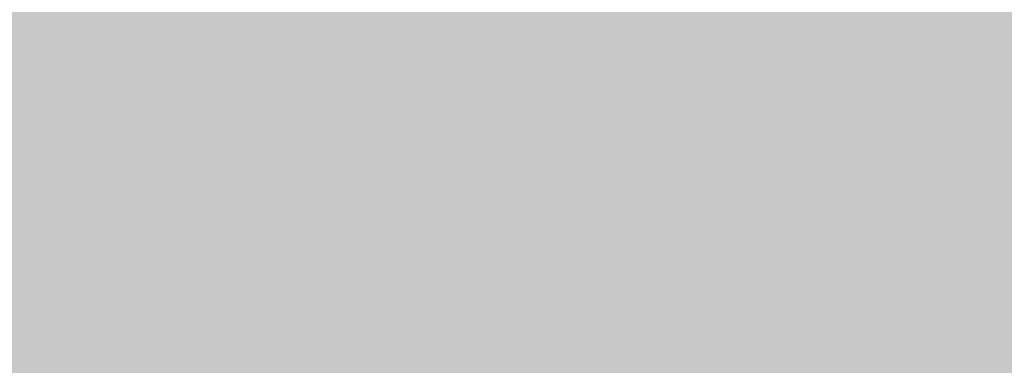
# Model space of a CAD drawing. Units: inches. Extents: x 2091 to 2899, y 967 to 2217.
# Tile 232 of 256: x 2203.4104 to 2203.7172, y 1152.3547 to 1152.4622. Entities that reach past the tile are written whole.
import ezdxf

# ---------------------------------------------------------------- set-up
doc = ezdxf.new("R2010")
doc.units = ezdxf.units.IN
doc.layers.add('A-WALL-PATT', color=141, linetype='Continuous', lineweight=13, true_color=0xadddf7)

msp = doc.modelspace()

# ---------------------------------------------------------------- hatches: boundary and pattern name
at = {"layer": 'A-WALL-PATT'}
h = msp.add_hatch(color=256, dxfattribs=at)
h.dxf.hatch_style = 1
h.paths.add_polyline_path([(2803.1436, 2050.91906), (2203.1436, 2050.91906), (2203.1436, 1090.91906), (2803.1436, 1090.91906)])
h.paths.add_polyline_path([(2635.79885, 1147.54046), (2674.52405, 1147.54046, 0.376086), (2678.52967, 1152.8802), (2678.52967, 1159.55647, 0.333335), (2674.52432, 1163.56185), (2674.52432, 1163.56185), (2674.52432, 1192.93439), (2635.80597, 1192.93439), (2597.08762, 1192.93439), (2597.08762, 1163.56185, 0.333335), (2593.08228, 1159.55647), (2593.08228, 1152.8802, 0.376086), (2597.08789, 1147.54046)], flags=0)
h.paths.add_polyline_path([(2436.01043, 1278.24078, 0.000483), (2435.95264, 1278.21503, -0.001328), (2435.93563, 1278.11169, -0.001711), (2436.11644, 1278.04076, 0.002185)], flags=0)
h.paths.add_polyline_path([(2794.1436, 1143.41906), (2794.1436, 1347.41906), (2543.37017, 1347.41906), (2543.37017, 1351.91906), (2794.1436, 1351.91906), (2794.1436, 1392.71355), (2793.9474, 1392.71355), (2793.9474, 1473.5369), (2794.1436, 1473.5369), (2794.1436, 1531.91906), (2650.1436, 1531.91906), (2650.1436, 1536.41906), (2794.1436, 1536.41906), (2794.1436, 1692.41906), (2609.37561, 1692.41906), (2609.37561, 1644.41906), (2604.87561, 1644.41906), (2604.87561, 1744.91906), (2609.37561, 1744.91906), (2609.37561, 1696.91906), (2794.1436, 1696.91906), (2794.1436, 1780.91906), (2609.6436, 1780.91906), (2493.87561, 1780.91906), (2493.87561, 1785.41906), (2609.6436, 1785.41906), (2794.1436, 1785.41906), (2794.1436, 1847.93882), (2793.95122, 1847.93882), (2793.95122, 1928.76217), (2794.1436, 1928.76217), (2794.1436, 1941.41906), (2614.1436, 1941.41906), (2614.1436, 1821.41906), (2609.6436, 1821.41906), (2609.6436, 1941.41906), (2392.1436, 1941.41906), (2392.1436, 1819.91906), (2387.6436, 1819.91906), (2387.6436, 1941.41906), (2212.1436, 1941.41906), (2212.1436, 1783.91906), (2392.1436, 1783.91906), (2392.1436, 1780.91906), (2212.1436, 1780.91906), (2212.1436, 1629.41906), (2387.6436, 1629.41906), (2387.6436, 1744.91906), (2392.1436, 1744.91906), (2392.1436, 1627.91906), (2317.1436, 1627.91906), (2317.1436, 1551.41906), (2317.1436, 1536.41906), (2459.38359, 1536.41906), (2459.38359, 1602.39648), (2463.88359, 1602.39648), (2463.88359, 1531.91906), (2456.6436, 1531.91906), (2456.6436, 1529.91906), (2452.1436, 1529.91906), (2452.1436, 1531.91906), (2312.6436, 1531.91906), (2312.6436, 1551.41906), (2306.1436, 1551.41906), (2306.1436, 1555.91906), (2308.1436, 1555.91906), (2308.1436, 1551.41906), (2312.6436, 1551.41906), (2312.6436, 1627.91906), (2212.1436, 1627.91906), (2212.1436, 1555.91906), (2270.1436, 1555.91906), (2270.1436, 1551.41906), (2212.1436, 1551.41906), (2212.1436, 1351.91906), (2272.1436, 1351.91906), (2272.1436, 1347.41906), (2212.1436, 1347.41906), (2212.1436, 1275.41906), (2308.1436, 1275.41906), (2308.1436, 1351.91906), (2452.1436, 1351.91906), (2452.1436, 1493.91906), (2456.6436, 1493.91906), (2456.6436, 1347.41906), (2312.6436, 1347.41906), (2312.6436, 1270.91906), (2212.1436, 1270.91906), (2212.1436, 1099.91906), (2281.23752, 1099.91906), (2282.87104, 1110.9138), (2282.00834, 1116.9966), (2278.55774, 1121.4204), (2268.20564, 1128.0562), (2272.08764, 1128.0562), (2273.81294, 1131.927), (2279.42034, 1134.6919), (2285.02784, 1135.2449), (2287.61584, 1137.4568), (2288.04714, 1138.0098), (2289.34114, 1140.7747), (2291.06654, 1139.6687), (2292.36054, 1135.2449), (2295.37984, 1136.9038), (2296.24254, 1135.7979), (2297.10524, 1133.033), (2300.12464, 1138.0098), (2303.14394, 1138.0098), (2304.43794, 1135.7979), (2303.14394, 1133.586), (2306.59464, 1134.6919), (2307.88874, 1133.033), (2310.90804, 1135.2449), (2313.92744, 1134.1389), (2315.62686, 1132.4271), (2308.32004, 1117.5496), (2290.20384, 1109.8079), (2288.90984, 1103.1721), (2289.27231, 1099.91906), (2434.91823, 1099.91906), (2431.59323, 1124.78806), (2429.93023, 1169.55306), (2430.92718, 1240.51969), (2435.65893, 1238.18613), (2437.13523, 1196.55406), (2438.79823, 1143.97306), (2442.67823, 1111.99806), (2446.55823, 1099.91906), (2794.1436, 1099.91906), (2794.1436, 1138.91906), (2548.03245, 1138.91906), (2548.03245, 1143.41906), (2548.03245, 1148.81906), (2546.66846, 1148.03156), (2528.68569, 1179.17862, 0.256256), (2512.03245, 1148.81906), (2512.03245, 1143.41906), (2512.03245, 1138.91906), (2507.53245, 1138.91906), (2507.53245, 1143.41906), (2507.53245, 1148.81906, 0.256256), (2490.8792, 1179.17862), (2472.89644, 1148.03156), (2471.53245, 1148.81906), (2471.53245, 1143.41906), (2467.03245, 1143.41906), (2467.03245, 1269.94579, 0.039061), (2460.90999, 1273.58006), (2467.03245, 1273.58006), (2467.03245, 1286.32536, 0.014511), (2465.21619, 1286.76191), (2467.03245, 1287.05258), (2467.03245, 1323.41906), (2471.53245, 1323.41906), (2471.53245, 1148.81906), (2489.53245, 1179.99597), (2490.89644, 1179.20847), (2490.8792, 1179.17862, -0.256256), (2507.53245, 1148.81906), (2507.53245, 1143.41906), (2512.03245, 1143.41906), (2512.03245, 1148.81906, -0.256256), (2528.68569, 1179.17862), (2528.66846, 1179.20847), (2530.03245, 1179.99597), (2548.03245, 1148.81906), (2548.03245, 1143.41906)], flags=16)
h.paths.add_polyline_path([(2607.76855, 1200.94508), (2607.76855, 1265.03063), (2597.08762, 1281.05201), (2619.78459, 1281.05201), (2627.79528, 1337.12686), (2635.79885, 1337.12686), (2643.81666, 1337.12686), (2651.82736, 1281.05201), (2674.52432, 1281.05201), (2663.8434, 1265.03063), (2663.8434, 1200.94508), (2635.80597, 1200.94508)], flags=0)
edge = h.paths.add_edge_path(flags=0)
edge.add_ellipse((13303.89622, 1272.99872), major_axis=(-10595.31304, 0), ratio=0.84230387009, start_angle=0.628237219, end_angle=0.6465541, ccw=False)
edge.add_ellipse((2711.70045, 1156.85268), major_axis=(2.21977, 0), ratio=0.8423039, start_angle=111.53524, end_angle=180.62824, ccw=False)
edge.add_ellipse((13303.15629, 1272.99872), major_axis=(-10593.02631, 0), ratio=0.84230386954, start_angle=0.528271472, end_angle=0.646554097, ccw=False)
edge.add_line((2710.7646, 1175.3333), (2710.12999, 1175.3333))
edge.add_ellipse((2710.12999, 1176.57978), major_axis=(1.47985, 0), ratio=0.8423039, start_angle=180, end_angle=270, ccw=False)
edge.add_line((2708.65014, 1176.57978), (2708.65014, 1200.78291))
edge.add_ellipse((2710.12999, 1200.78291), major_axis=(1.47985, 0), ratio=0.8423039, start_angle=90, end_angle=180, ccw=False)
edge.add_line((2710.12999, 1202.02939), (2710.46508, 1202.02939))
edge.add_ellipse((13303.15629, 1272.99872), major_axis=(-10593.02631, 0), ratio=0.84230386954, start_angle=-0.090229089, end_angle=0.383866779, ccw=False)
edge.add_ellipse((2710.12999, 1290.92703), major_axis=(-1.47985, 0), ratio=0.8423039, start_angle=0, end_angle=90, ccw=False)
edge.add_line((2708.65014, 1290.92703), (2708.65014, 1315.13017))
edge.add_ellipse((2710.12999, 1315.13017), major_axis=(-1.47985, 0), ratio=0.8423039, start_angle=-90, end_angle=0, ccw=False)
edge.add_line((2710.12999, 1316.37665), (2710.70631, 1316.37665))
edge.add_ellipse((3238.40172, 1296.28957), major_axis=(528.234, 0), ratio=0.84230387, start_angle=176.3495724, end_angle=177.8200497, ccw=False)
edge.add_ellipse((2775.06304, 1071.4507), major_axis=(313.30776, 0), ratio=0.84230387, start_angle=102.1259656, end_angle=103.780529, ccw=False)
edge.add_ellipse((2775.06304, 1078.3057), major_axis=(-305.30289, 0), ratio=0.84230387, start_angle=-79.790461, end_angle=-77.5553727, ccw=False)
edge.add_ellipse((2695.14177, 1541.97538), major_axis=(-250.96022, 0), ratio=0.84230387, start_angle=99.256566, end_angle=102.5549326)
edge.add_line((2741.41033, 1334.21426), (2747.13255, 1337.37848))
edge.add_ellipse((2747.53862, 1336.85748), major_axis=(-0.73992, 0), ratio=0.842304, start_angle=270, end_angle=307.93313, ccw=False)
edge.add_ellipse((2747.53862, 1336.85748), major_axis=(-0.73992, 0), ratio=0.842304, start_angle=232.06687, end_angle=270, ccw=False)
edge.add_line((2747.94469, 1337.37848), (2753.66691, 1334.21426))
edge.add_ellipse((2799.93547, 1541.97538), major_axis=(250.96022, 0), ratio=0.84230387, start_angle=257.4450674, end_angle=260.743434)
edge.add_ellipse((2720.01419, 1078.3057), major_axis=(305.30289, 0), ratio=0.84230387, start_angle=77.5553727, end_angle=79.790461, ccw=False)
edge.add_ellipse((2720.01419, 1071.4507), major_axis=(-313.30776, 0), ratio=0.84230387, start_angle=256.219471, end_angle=257.8740344, ccw=False)
edge.add_ellipse((2256.67551, 1296.28957), major_axis=(-528.234, 0), ratio=0.84230387, start_angle=182.1799503, end_angle=183.6504276, ccw=False)
edge.add_line((2784.37092, 1316.37665), (2784.94725, 1316.37665))
edge.add_ellipse((2784.94725, 1315.13017), major_axis=(1.47985, 0), ratio=0.8423039, start_angle=0, end_angle=90, ccw=False)
edge.add_line((2786.42709, 1315.13017), (2786.42709, 1290.92703))
edge.add_ellipse((2784.94725, 1290.92703), major_axis=(1.47985, 0), ratio=0.8423039, start_angle=270, end_angle=360, ccw=False)
edge.add_ellipse((-7808.07906, 1272.99872), major_axis=(10593.02631, 0), ratio=0.84230386954, start_angle=-0.383866779, end_angle=0.090229089, ccw=False)
edge.add_line((2784.61216, 1202.02939), (2784.94725, 1202.02939))
edge.add_ellipse((2784.94725, 1200.78291), major_axis=(1.47985, 0), ratio=0.8423039, start_angle=0, end_angle=90, ccw=False)
edge.add_line((2786.42709, 1200.78291), (2786.42709, 1176.57978))
edge.add_ellipse((2784.94725, 1176.57978), major_axis=(-1.47985, 0), ratio=0.8423039, start_angle=90, end_angle=180, ccw=False)
edge.add_line((2784.94725, 1175.3333), (2784.31264, 1175.3333))
edge.add_ellipse((-7808.07906, 1272.99872), major_axis=(10593.02631, 0), ratio=0.84230386954, start_angle=-0.618643196, end_angle=-0.528271472, ccw=False)
edge.add_ellipse((2783.37678, 1156.85268), major_axis=(-2.21977, 0), ratio=0.8423039, start_angle=179.37176, end_angle=248.46476, ccw=False)
edge.add_ellipse((-7808.81898, 1272.99872), major_axis=(-10595.31304, 0), ratio=0.84230386576, start_angle=179.353445923, end_angle=179.371762803, ccw=False)
edge.add_ellipse((2780.2973, 1153.50079), major_axis=(-5.24643, 0), ratio=0.8423039, start_angle=90, end_angle=179.35345, ccw=False)
edge.add_line((2780.2973, 1149.08171), (2714.77993, 1149.08171))
edge.add_ellipse((2714.77993, 1153.50079), major_axis=(5.24643, 0), ratio=0.8423039, start_angle=180.64655, end_angle=270, ccw=False)
edge = h.paths.add_edge_path(flags=0)
edge.add_line((2718.18737, 1151.00783), (2718.18737, 1170.47236))
edge.add_ellipse((2721.14706, 1170.47236), major_axis=(-2.95969, 0), ratio=0.8423039, start_angle=-90, end_angle=0, ccw=False)
edge.add_line((2721.14706, 1172.96532), (2773.93017, 1172.96532))
edge.add_ellipse((2773.93017, 1170.47236), major_axis=(-2.95969, 0), ratio=0.8423039, start_angle=180, end_angle=270, ccw=False)
edge.add_line((2776.88987, 1170.47236), (2776.88987, 1151.00783))
edge.add_line((2776.88987, 1151.00783), (2718.18737, 1151.00783))
edge = h.paths.add_edge_path(flags=0)
edge.add_line((2718.18737, 1180.23415), (2718.18737, 1199.05783))
edge.add_ellipse((2747.53862, 1320.39864), major_axis=(147.01792, 0), ratio=0.84230387, start_angle=256.4018653, end_angle=283.5981347)
edge.add_line((2776.88987, 1199.05783), (2776.88987, 1180.23415))
edge.add_ellipse((2747.53862, 1301.57496), major_axis=(147.01792, 0), ratio=0.84230387, start_angle=256.4018653, end_angle=283.5981347, ccw=False)
edge = h.paths.add_edge_path(flags=0)
edge.add_ellipse((13303.15629, 1272.99872), major_axis=(-10591.54646, 0), ratio=0.84230386955, start_angle=0.055594314, end_angle=0.377764194, ccw=False)
edge.add_line((2711.61686, 1262.72171), (2715.66741, 1249.4954))
edge.add_ellipse((6413.89196, 1241.69192), major_axis=(-3698.23616, 0), ratio=0.8423038695, start_angle=-0.12089737, end_angle=0.36407635)
edge.add_line((2715.76104, 1218.19245), (2711.93431, 1203.16736))
edge = h.paths.add_edge_path(flags=0)
edge.add_line((2718.18737, 1251.07457), (2716.00249, 1267.45044))
edge.add_ellipse((2742.15117, 1202.18954), major_axis=(81.77258, 0), ratio=0.84230387, start_angle=94.277421, end_angle=111.8349538, ccw=False)
edge.add_line((2737.00975, 1270.93063), (2758.06748, 1270.93063))
edge.add_ellipse((2752.92606, 1202.18954), major_axis=(81.77258, 0), ratio=0.84230387, start_angle=68.1650462, end_angle=85.722579, ccw=False)
edge.add_line((2779.07475, 1267.45044), (2776.88987, 1251.07457))
edge.add_ellipse((2750.33806, 1187.88536), major_axis=(79.57966, 0), ratio=0.84230387, start_angle=67.2080851, end_angle=85.1299304)
edge.add_line((2756.03466, 1254.74366), (2739.04258, 1254.74366))
edge.add_ellipse((2744.73917, 1187.88536), major_axis=(79.57966, 0), ratio=0.84230387, start_angle=94.8700696, end_angle=112.7919149)
edge = h.paths.add_edge_path(flags=0)
edge.add_line((2783.14293, 1203.16736), (2779.31619, 1218.19245))
edge.add_ellipse((-918.81473, 1241.69192), major_axis=(3698.23616, 0), ratio=0.8423038695, start_angle=-0.36407635, end_angle=0.12089737)
edge.add_line((2779.40983, 1249.4954), (2783.46037, 1262.72171))
edge.add_ellipse((-7808.07906, 1272.99872), major_axis=(-10591.54646, 0), ratio=0.84230386954, start_angle=179.622235806, end_angle=179.944405687, ccw=False)
edge = h.paths.add_edge_path(flags=0)
edge.add_ellipse((2734.20089, 1286.69044), major_axis=(-0.35661, 6.34008), ratio=0.6038336, start_angle=89.002014, end_angle=253.657408, ccw=False)
edge.add_line((2730.369, 1286.54181), (2730.369, 1301.35198))
edge.add_line((2730.369, 1301.35198), (2735.91331, 1305.2148))
edge.add_ellipse((2736.38492, 1304.73456), major_axis=(0.73992, 0), ratio=0.842304, start_angle=90, end_angle=134.48021, ccw=False)
edge.add_line((2736.38492, 1305.3578), (2738.03278, 1305.3578))
edge.add_line((2738.03278, 1305.3578), (2738.03278, 1307.70793))
edge.add_ellipse((2794.20164, 1307.70793), major_axis=(56.16886, 0), ratio=0.84230387, start_angle=150.56143, end_angle=180, ccw=False)
edge.add_ellipse((2700.87559, 1307.70793), major_axis=(-56.16886, 0), ratio=0.84230387, start_angle=180, end_angle=209.43857, ccw=False)
edge.add_line((2757.04445, 1307.70793), (2757.04445, 1305.3578))
edge.add_line((2757.04445, 1305.3578), (2758.69232, 1305.3578))
edge.add_ellipse((2758.69232, 1304.73456), major_axis=(-0.73992, 0), ratio=0.842304, start_angle=225.51979, end_angle=270, ccw=False)
edge.add_line((2759.16392, 1305.2148), (2764.70823, 1301.35198))
edge.add_line((2764.70823, 1301.35198), (2764.70823, 1286.54181))
edge.add_ellipse((2760.87634, 1286.69044), major_axis=(0.35661, 6.34008), ratio=0.6038336, start_angle=106.342592, end_angle=270.997986, ccw=False)
edge.add_line((2757.04445, 1285.79709), (2757.04445, 1307.70793))
edge.add_ellipse((2700.87559, 1307.70793), major_axis=(-56.16886, 0), ratio=0.84230387, start_angle=180, end_angle=209.43857)
edge.add_ellipse((2794.20164, 1307.70793), major_axis=(56.16886, 0), ratio=0.84230387, start_angle=150.56143, end_angle=180)
edge.add_line((2738.03278, 1307.70793), (2738.03278, 1285.79709))
h.paths.add_polyline_path([(2417.81227, 1104.4497), (2413.49227, 1102.5297), (2410.61227, 1103.9697), (2409.17227, 1106.3697), (2407.25227, 1107.3297), (2406.29227, 1109.7297), (2405.33227, 1114.0497), (2405.33227, 1117.8897), (2406.29227, 1120.1297), (2407.25227, 1119.8097), (2408.84832, 1118.32766), (2410.17395, 1119.42417), (2410.21127, 1120.4057), (2411.04073, 1121.41905), (2410.69927, 1119.8587), (2410.17395, 1119.42417), (2410.08845, 1117.17611), (2411.13284, 1116.20632), (2413.97227, 1119.3297), (2416.85227, 1120.7697), (2416.86972, 1120.79878), (2417.03507, 1119.40512), (2417.89621, 1118.14338), (2418.29227, 1118.3697), (2419.54445, 1120.03927), (2419.36092, 1118.38749), (2419.03211, 1119.35615), (2418.39894, 1118.51193), (2419.25227, 1114.5297), (2418.79409, 1107.19879)], flags=0)
h.paths.add_polyline_path([(2508.87017, 1347.41906), (2508.37017, 1347.41906), (2508.37017, 1351.91906), (2508.87017, 1351.91906)], flags=0)
h.paths.add_polyline_path([(2473.37017, 1347.41906), (2472.37017, 1347.41906), (2467.87017, 1347.41906), (2467.87017, 1455.41906), (2472.37017, 1455.41906), (2472.37017, 1352.41906), (2473.37017, 1352.41906)], flags=0)
h.paths.add_polyline_path([(2352.10624, 1217.4462), (2349.22624, 1218.8862), (2347.78624, 1221.2862), (2345.86624, 1222.2462), (2344.90624, 1224.6462), (2343.94624, 1228.9662), (2343.94624, 1232.8062), (2344.90624, 1235.0462), (2345.86624, 1234.7262), (2347.46229, 1233.24415), (2348.78792, 1234.34066), (2348.82524, 1235.3222), (2349.6547, 1236.33555), (2349.31324, 1234.7752), (2348.78792, 1234.34066), (2348.70242, 1232.0926), (2349.74681, 1231.12282), (2352.58624, 1234.2462), (2355.46624, 1235.6862), (2355.48369, 1235.71528), (2355.64904, 1234.32161), (2356.51018, 1233.05988), (2356.90624, 1233.2862), (2358.15842, 1234.95576), (2357.97489, 1233.30398), (2357.64608, 1234.27264), (2357.01291, 1233.42842), (2357.86624, 1229.4462), (2357.40806, 1222.11529), (2356.42624, 1219.3662)], flags=0)
h.paths.add_polyline_path([(2348.2968, 1112.22442), (2347.0138, 1112.31042), (2345.5298, 1114.12742), (2345.7318, 1115.85842), (2346.8118, 1116.98242), (2346.8118, 1114.64642), (2345.8668, 1114.21442), (2346.8798, 1114.30042)], flags=0)
h.paths.add_polyline_path([(2347.0138, 1110.92642), (2346.2718, 1110.49342), (2346.6098, 1111.18642)], flags=0)
h.paths.add_polyline_path([(2345.8668, 1118.19442), (2345.5298, 1117.32942), (2343.7078, 1118.02142), (2344.3828, 1118.62642)], flags=0)
h.paths.add_polyline_path([(2346.6768, 1109.28242), (2346.0698, 1108.07142), (2345.8668, 1110.06142)], flags=0)
h.paths.add_polyline_path([(2345.0568, 1119.75142), (2343.6398, 1119.75142), (2343.9778, 1121.13542)], flags=0)
h.paths.add_polyline_path([(2345.2598, 1116.55042), (2345.1248, 1115.85842), (2344.9218, 1115.68542), (2344.7198, 1116.37742)], flags=0)
h.paths.add_polyline_path([(2345.6648, 1112.31042), (2345.4618, 1111.53242), (2344.0448, 1111.96442), (2344.6518, 1112.57042)], flags=0)
h.paths.add_polyline_path([(2345.1918, 1113.34942), (2344.4498, 1113.86842), (2344.7198, 1114.38742)], flags=0)
h.paths.add_polyline_path([(2344.6518, 1116.80942), (2344.1798, 1115.68542), (2344.6518, 1115.33942), (2343.9098, 1114.90642), (2343.0328, 1115.94442), (2343.6398, 1116.46342)], flags=0)
h.paths.add_polyline_path([(2345.8668, 1106.68642), (2344.9898, 1105.56242), (2344.5168, 1106.60042)], flags=0)
h.paths.add_polyline_path([(2344.8548, 1110.06142), (2344.5168, 1109.28242), (2344.1128, 1109.71542)], flags=0)
h.paths.add_polyline_path([(2344.0448, 1113.52242), (2343.4378, 1113.08942), (2342.7628, 1113.95442)], flags=0)
h.paths.add_polyline_path([(2344.3148, 1111.01242), (2342.9648, 1110.32042), (2342.9648, 1111.09942)], flags=0)
h.paths.add_polyline_path([(2345.1248, 1104.69742), (2344.5848, 1103.74542), (2344.4498, 1104.26442)], flags=0)
h.paths.add_polyline_path([(2342.8298, 1121.22242), (2341.7498, 1120.53042), (2340.5358, 1121.04942), (2340.1308, 1121.82842), (2340.6708, 1122.95242), (2341.1428, 1121.82842), (2341.6148, 1122.00142)], flags=0)
h.paths.add_polyline_path([(2342.9648, 1119.75142), (2343.0328, 1118.45342), (2342.0878, 1118.02142), (2342.0198, 1119.49142)], flags=0)
h.paths.add_polyline_path([(2342.6948, 1116.89642), (2341.9528, 1116.63642), (2342.0198, 1117.32942)], flags=0)
h.paths.add_polyline_path([(2343.0328, 1112.22442), (2342.0198, 1111.79142), (2341.5478, 1112.22442), (2342.3578, 1113.34942)], flags=0)
h.paths.add_polyline_path([(2343.7748, 1104.43742), (2342.6278, 1102.88042), (2342.6948, 1104.61042), (2343.4378, 1105.12942)], flags=0)
h.paths.add_polyline_path([(2342.0198, 1115.07942), (2340.8058, 1115.51242), (2340.9408, 1116.37742)], flags=0)
h.paths.add_polyline_path([(2341.4808, 1120.09742), (2341.4808, 1119.40542), (2341.0758, 1119.57842), (2341.1428, 1120.09742)], flags=0)
h.paths.add_polyline_path([(2341.8178, 1114.47342), (2340.9408, 1113.08942), (2340.8058, 1114.56042)], flags=0)
h.paths.add_polyline_path([(2341.1428, 1118.54042), (2340.9408, 1116.98242), (2339.0508, 1117.67542), (2339.0508, 1118.62642)], flags=0)
h.paths.add_polyline_path([(2342.6948, 1101.66842), (2341.9528, 1101.84142), (2342.5598, 1102.36142)], flags=0)
h.paths.add_polyline_path([(2340.3328, 1119.66542), (2338.4438, 1119.57842), (2337.9038, 1120.35742), (2339.6578, 1120.61642)], flags=0)
h.paths.add_polyline_path([(2340.3328, 1115.33942), (2340.0628, 1113.69542), (2339.3878, 1115.33942)], flags=0)
h.paths.add_polyline_path([(2341.8178, 1103.83142), (2341.5478, 1102.88042), (2341.1428, 1103.65842)], flags=0)
h.paths.add_polyline_path([(2339.0508, 1122.86642), (2337.2958, 1121.82842), (2337.0938, 1123.12542), (2337.7688, 1123.81842)], flags=0)
h.paths.add_polyline_path([(2339.1178, 1121.74142), (2338.8478, 1121.22242), (2338.1738, 1121.04942), (2338.3758, 1121.56842)], flags=0)
h.paths.add_polyline_path([(2339.1858, 1119.31942), (2338.6458, 1118.71342), (2338.2408, 1118.10742), (2338.2408, 1118.88642)], flags=0)
h.paths.add_polyline_path([(2341.1428, 1101.92842), (2340.6028, 1101.23642), (2340.0628, 1101.84142), (2340.6028, 1102.36142)], flags=0)
h.paths.add_polyline_path([(2337.6338, 1117.76142), (2336.6208, 1118.28042), (2337.2958, 1118.97242)], flags=0)
h.paths.add_polyline_path([(2336.8238, 1119.57842), (2334.7988, 1118.97242), (2335.2038, 1120.35742), (2336.5538, 1120.87642)], flags=0)
h.paths.add_polyline_path([(2339.1178, 1100.45742), (2337.3638, 1100.54342), (2336.7558, 1101.23642)], flags=0)
h.paths.add_polyline_path([(2336.3508, 1122.43342), (2336.0138, 1121.91442), (2334.9338, 1122.43342), (2334.5288, 1123.47142), (2335.7438, 1122.77942)], flags=0)
h.paths.add_polyline_path([(2334.7318, 1120.87642), (2334.2588, 1120.35742), (2334.0568, 1120.78942), (2334.5968, 1121.30842)], flags=0)
h.paths.add_polyline_path([(2334.4618, 1122.17442), (2332.5718, 1121.30842), (2331.3568, 1122.17442), (2332.0998, 1122.86642)], flags=0)
h.paths.add_polyline_path([(2334.2588, 1118.54042), (2333.3818, 1118.45342), (2333.6518, 1119.31942)], flags=0)
h.paths.add_polyline_path([(2335.5418, 1102.27442), (2334.1918, 1102.62042), (2335.2718, 1103.31242)], flags=0)
h.paths.add_polyline_path([(2332.7068, 1119.66542), (2331.6948, 1120.44342), (2332.5048, 1120.78942)], flags=0)
h.paths.add_polyline_path([(2334.7318, 1101.14942), (2333.5168, 1101.58242), (2333.9888, 1101.75542)], flags=0)
h.paths.add_polyline_path([(2332.6398, 1116.63642), (2331.0868, 1116.29042), (2331.9648, 1118.19442)], flags=0)
h.paths.add_polyline_path([(2330.7498, 1121.56842), (2330.2768, 1120.27042), (2328.5228, 1119.31942), (2328.9948, 1121.04942)], flags=0)
h.paths.add_polyline_path([(2330.7498, 1118.62642), (2330.0078, 1117.50242), (2329.8728, 1118.02142)], flags=0)
h.paths.add_polyline_path([(2332.0998, 1102.36142), (2330.5468, 1102.01442), (2331.6948, 1102.96642)], flags=0)
h.paths.add_polyline_path([(2329.5348, 1113.60842), (2329.0628, 1112.31042), (2328.5898, 1113.34942)], flags=0)
h.paths.add_polyline_path([(2328.3878, 1117.84842), (2327.5098, 1116.55042), (2327.1728, 1117.76142)], flags=0)
h.paths.add_polyline_path([(2329.7378, 1106.51342), (2329.5348, 1105.30242), (2328.2528, 1106.08142)], flags=0)
h.paths.add_polyline_path([(2328.6578, 1114.38742), (2328.0498, 1114.12742), (2328.3198, 1114.90642)], flags=0)
h.paths.add_polyline_path([(2328.3198, 1112.22442), (2327.1058, 1112.13742), (2326.7008, 1112.65642)], flags=0)
h.paths.add_polyline_path([(2326.9028, 1115.25242), (2326.7008, 1114.12742), (2325.2158, 1113.60842), (2326.0928, 1115.33942)], flags=0)
h.paths.add_polyline_path([(2326.6328, 1108.33042), (2326.0928, 1107.37942), (2325.8908, 1108.50342), (2326.4978, 1109.10942)], flags=0)
h.paths.add_polyline_path([(2615.1436, 1531.91906), (2609.6436, 1531.91906), (2609.6436, 1620.41906), (2614.1436, 1620.41906), (2614.1436, 1536.41906), (2615.1436, 1536.41906)], flags=0)
h.paths.add_polyline_path([(2545.1436, 1563.41906), (2464.1436, 1563.41906), (2464.1436, 1632.41906), (2509.1436, 1632.41906), (2509.1436, 1627.91906), (2509.1436, 1603.91906), (2468.6436, 1603.91906), (2468.6436, 1567.91906), (2540.6436, 1567.91906), (2540.6436, 1591.91906), (2545.1436, 1591.91906)], flags=0)
h.paths.add_polyline_path([(2388.96905, 1549.98573), (2357.43418, 1549.98573), (2357.43418, 1623.36078), (2399.36278, 1623.36078), (2435.68947, 1623.36078), (2435.59255, 1602.55927), (2435.59255, 1602.39648), (2388.96905, 1602.39648)], flags=0)
h.paths.add_polyline_path([(2388.88063, 1555.80915), (2374.90443, 1555.80915), (2374.90443, 1600.57156), (2374.90443, 1615.45765), (2406.35088, 1615.45765), (2406.35088, 1618.93943), (2412.17429, 1615.45765), (2406.35088, 1611.97586), (2406.35088, 1615.45765), (2388.88063, 1615.45765)], flags=0)
h.paths.add_polyline_path([(2568.87561, 1644.41906), (2453.37561, 1644.41906), (2453.37561, 1785.41906), (2457.87561, 1785.41906), (2457.87561, 1648.91906), (2568.87561, 1648.91906)], flags=0)
h.paths.add_polyline_path([(2212.1436, 1945.91906), (2212.1436, 2041.91906), (2794.1436, 2041.91906), (2794.1436, 1945.91906)], flags=16)
h.paths.add_polyline_path([(2271.08273, 1964.31724), (2776.85297, 1964.31724), (2776.85297, 2037.16962), (2271.08273, 2037.16962)], flags=8)
h.paths.add_polyline_path([(2380.64929, 1536.82414), (2461.04081, 1536.82414), (2461.04081, 1554.65259), (2380.64929, 1554.65259)], flags=8)
h.paths.add_polyline_path([(2240.75571, 1609.72545), (2309.18583, 1609.72545), (2309.18583, 1617.6982), (2240.75571, 1617.6982)], flags=8)
h.paths.add_polyline_path([(2212.67726, 1313.5041), (2282.59152, 1313.5041), (2282.59152, 1322.74524), (2212.67726, 1322.74524)], flags=8)
h.paths.add_polyline_path([(2457.11198, 1114.77857), (2558.48158, 1114.77857), (2558.48158, 1142.21968), (2457.11198, 1142.21968)], flags=8)
h.paths.add_polyline_path([(2473.44234, 1273.01007), (2604.64123, 1273.01007), (2604.64123, 1318.34693), (2473.44234, 1318.34693)], flags=8)
h.paths.add_polyline_path([(2638.8763, 1626.97743), (2684.25037, 1627.97674), (2684.03848, 1637.59749), (2638.66442, 1636.59819)], flags=8)
h.paths.add_polyline_path([(2537.59055, 1453.79345), (2628.38955, 1453.79345), (2628.38955, 1475.34481), (2537.59055, 1475.34481)], flags=8)
h.paths.add_polyline_path([(2504.13764, 1714.6324), (2554.64719, 1714.6324), (2554.64719, 1730.23771), (2504.13764, 1730.23771)], flags=8)
h.paths.add_polyline_path([(2487.50118, 1575.65187), (2535.09712, 1575.65187), (2535.09712, 1598.37765), (2487.50118, 1598.37765)], flags=8)
h.paths.add_polyline_path([(2709.0994, 1735.71028), (2740.0166, 1735.71028), (2740.0166, 1749.93764), (2709.0994, 1749.93764)], flags=8)
h.paths.add_polyline_path([(2442.43842, 1792.17166), (2564.72884, 1792.17166), (2564.72884, 1842.00016), (2442.43842, 1842.00016)], flags=8)
h.paths.add_polyline_path([(2655.8158, 1809.64408), (2789.52014, 1806.6938), (2790.08498, 1832.29164), (2656.38064, 1835.24192)], flags=8)
h.paths.add_polyline_path([(2234.8427, 1797.72014), (2368.59285, 1794.76885), (2369.16072, 1820.50413), (2235.41056, 1823.45542)], flags=8)
h.paths.add_polyline_path([(2245.13847, 1644.00633), (2398.42773, 1640.6239), (2398.99484, 1666.32482), (2245.70557, 1669.70725)], flags=8)
h.paths.add_polyline_path([(2306.14285, 1431.16852), (2413.76831, 1428.79369), (2414.33315, 1454.39153), (2306.70768, 1456.76636)], flags=8)
h.paths.add_polyline_path([(2306.83458, 1458.23314), (2393.38048, 1456.32345), (2393.93281, 1481.35436), (2307.38691, 1483.26405)], flags=8)

doc.saveas('drawing.dxf')
